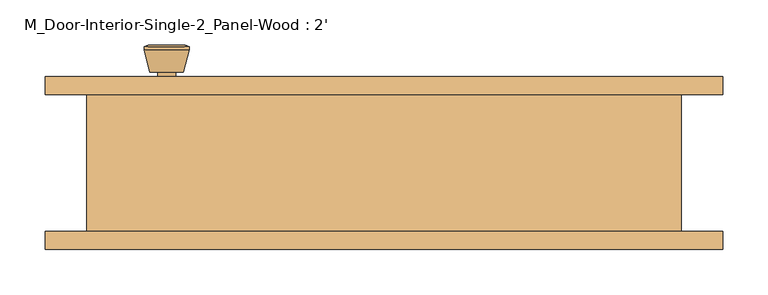
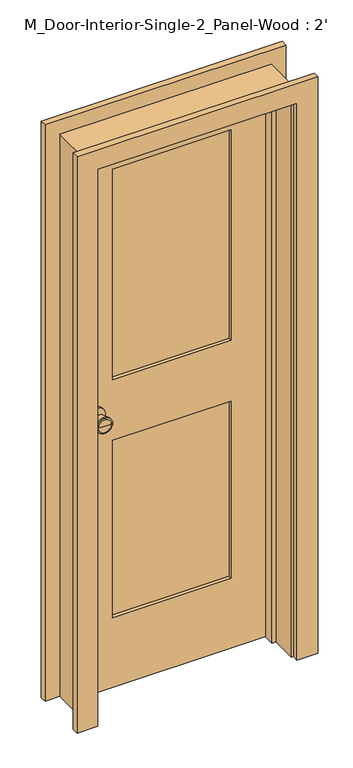
"""IFC4 building model written with IfcOpenShell, lengths in millimetres: door geometry, M_Door-Interior-Single-2_Panel-Wood : 2'."""

from ifc_helpers import new_model, si_unit, point, frame, frame_2d, origin, place, context, project, spatial, polyline, circle_curve, trimmed, segment, composite_curve, outline, extrude, faceted_brep, source, transform, mapped, element, save
from ifc_brep_helpers import plane_surface, cylinder_surface, revolved_surface, advanced_brep


def m_door_interior_single_2_panel_wood_2_8c5b34de(model_context):
    return source(origin(), model_context, "Body", "SolidModel", [
        advanced_brep(
        [(-241.3, 32.025, 914.4), (-231.3, 32.025, 914.4), (-251.3, 32.025, 914.4), (-220.8241324, -16.975, 914.4), (-241.3, -16.975, 914.4), (-261.7758676, -16.975, 914.4), (-216.3, -15.1471319, 914.4), (-266.3, -15.1471319, 914.4), (-216.3, -11.6834537, 914.4), (-266.3, -11.6834537, 914.4), (-222.663764, 13.025, 914.4), (-259.936236, 13.025, 914.4), (-231.3, 13.025, 914.4), (-251.3, 13.025, 914.4)],
        [
            (0, 1),
            (1, 2, circle_curve(frame((-241.3, 32.025, 914.4), z_axis=(0.0, 1.0, 0.0), x_axis=(-1.0, 0.0, 0.0)), 10.0)),
            (2, 0),
            (2, 1, circle_curve(frame((-241.3, 32.025, 914.4), z_axis=(0.0, 1.0, 0.0), x_axis=(-1.0, 0.0, 0.0)), 10.0)),
            (3, 4),
            (4, 5),
            (5, 3, circle_curve(frame((-241.3, -16.975, 914.4), z_axis=(0.0, -1.0, 0.0), x_axis=(-1.0, 0.0, 0.0)), 20.4758676)),
            (3, 5, circle_curve(frame((-241.3, -16.975, 914.4), z_axis=(0.0, -1.0, 0.0), x_axis=(-1.0, 0.0, 0.0)), 20.4758676)),
            (6, 3),
            (5, 7),
            (7, 6, circle_curve(frame((-241.3, -15.1471319, 914.4), z_axis=(0.0, -1.0, 0.0), x_axis=(-1.0, 0.0, 0.0)), 25.0)),
            (6, 7, circle_curve(frame((-241.3, -15.1471319, 914.4), z_axis=(0.0, -1.0, 0.0), x_axis=(-1.0, 0.0, 0.0)), 25.0)),
            (8, 6),
            (7, 9),
            (9, 8, circle_curve(frame((-241.3, -11.6834537, 914.4), z_axis=(0.0, -1.0, 0.0), x_axis=(-1.0, 0.0, 0.0)), 25.0)),
            (8, 9, circle_curve(frame((-241.3, -11.6834537, 914.4), z_axis=(0.0, -1.0, 0.0), x_axis=(-1.0, 0.0, 0.0)), 25.0)),
            (10, 8),
            (9, 11),
            (11, 10, circle_curve(frame((-241.3, 13.025, 914.4), z_axis=(0.0, -1.0, 0.0), x_axis=(-1.0, 0.0, 0.0)), 18.636236)),
            (10, 11, circle_curve(frame((-241.3, 13.025, 914.4), z_axis=(0.0, -1.0, 0.0), x_axis=(-1.0, 0.0, 0.0)), 18.636236)),
            (12, 10),
            (11, 13),
            (13, 12, circle_curve(frame((-241.3, 13.025, 914.4), z_axis=(0.0, -1.0, 0.0), x_axis=(-1.0, 0.0, 0.0)), 10.0)),
            (12, 13, circle_curve(frame((-241.3, 13.025, 914.4), z_axis=(0.0, -1.0, 0.0), x_axis=(-1.0, 0.0, 0.0)), 10.0)),
            (1, 12),
            (13, 2),
        ],
        [
            plane_surface(frame((-241.3, 32.025, 914.4), z_axis=(0.0, 1.0, 0.0), x_axis=(-1.0, 0.0, 0.0))),
            plane_surface(frame((-241.3, -16.975, 914.4), z_axis=(0.0, -1.0, 0.0), x_axis=(-1.0, 0.0, 0.0))),
            revolved_surface(polyline([(-261.7758676, -16.975, 914.4), (-266.3, -15.1471319, 914.4)]), (-241.3, 32.025, 914.4), (0.0, 1.0, 0.0)),
            cylinder_surface(frame((-241.3, 32.025, 914.4), z_axis=(0.0, 1.0, 0.0), x_axis=(-1.0, 0.0, 0.0)), 25.0),
            revolved_surface(polyline([(-266.3, -11.6834537, 914.4), (-259.936236, 13.025, 914.4)]), (-241.3, 32.025, 914.4), (0.0, 1.0, 0.0)),
            plane_surface(frame((-241.3, 13.025, 914.4), z_axis=(0.0, 1.0, 0.0), x_axis=(-1.0, 0.0, 0.0))),
            cylinder_surface(frame((-241.3, 32.025, 914.4), z_axis=(0.0, 1.0, 0.0), x_axis=(-1.0, 0.0, 0.0)), 10.0),
        ],
        [
            (0, [[1, 2, 3]]),
            (0, [[-3, 4, -1]]),
            (1, [[5, 6, 7]]),
            (1, [[-6, -5, 8]]),
            (2, [[9, -7, 10, 11]]),
            (2, [[-10, -8, -9, 12]]),
            (3, [[13, -11, 14, 15]]),
            (3, [[-14, -12, -13, 16]]),
            (4, [[17, -15, 18, 19]]),
            (4, [[-18, -16, -17, 20]]),
            (5, [[21, -19, 22, 23]]),
            (5, [[-22, -20, -21, 24]]),
            (6, [[25, -23, 26, -2]]),
            (6, [[-26, -24, -25, -4]]),
        ],
    ),
        extrude(outline(composite_curve([segment(trimmed(circle_curve(frame_2d((914.4, -241.3)), 30.0), [point((914.4, -271.3))], [point((914.4, -211.3))], False, "CARTESIAN"), True, "CONTINUOUS"), segment(trimmed(circle_curve(frame_2d((914.4, -241.3)), 30.0), [point((914.4, -211.3))], [point((914.4, -271.3))], False, "CARTESIAN"), True, "CONTINUOUS")], self_intersect=False)), frame((0.0, 32.025, 0.0), z_axis=(0.0, 1.0, 0.0), x_axis=(0.0, 0.0, 1.0)), (0.0, 0.0, 1.0), 6.0),
        advanced_brep(
        [(-241.3, 79.025, 914.4), (-251.3, 79.025, 914.4), (-231.3, 79.025, 914.4), (-220.8241324, 128.025, 914.4), (-261.7758676, 128.025, 914.4), (-241.3, 128.025, 914.4), (-216.3, 126.1971319, 914.4), (-266.3, 126.1971319, 914.4), (-216.3, 122.7334537, 914.4), (-266.3, 122.7334537, 914.4), (-222.663764, 98.025, 914.4), (-259.936236, 98.025, 914.4), (-231.3, 98.025, 914.4), (-251.3, 98.025, 914.4)],
        [
            (0, 1),
            (1, 2, circle_curve(frame((-241.3, 79.025, 914.4), z_axis=(0.0, -1.0, 0.0), x_axis=(-1.0, 0.0, 0.0)), 10.0)),
            (2, 0),
            (2, 1, circle_curve(frame((-241.3, 79.025, 914.4), z_axis=(0.0, -1.0, 0.0), x_axis=(-1.0, 0.0, 0.0)), 10.0)),
            (3, 4, circle_curve(frame((-241.3, 128.025, 914.4), z_axis=(0.0, 1.0, 0.0), x_axis=(-1.0, 0.0, 0.0)), 20.4758676)),
            (4, 5),
            (5, 3),
            (4, 3, circle_curve(frame((-241.3, 128.025, 914.4), z_axis=(0.0, 1.0, 0.0), x_axis=(-1.0, 0.0, 0.0)), 20.4758676)),
            (6, 7, circle_curve(frame((-241.3, 126.1971319, 914.4), z_axis=(0.0, 1.0, 0.0), x_axis=(-1.0, 0.0, 0.0)), 25.0)),
            (7, 4),
            (3, 6),
            (7, 6, circle_curve(frame((-241.3, 126.1971319, 914.4), z_axis=(0.0, 1.0, 0.0), x_axis=(-1.0, 0.0, 0.0)), 25.0)),
            (8, 9, circle_curve(frame((-241.3, 122.7334537, 914.4), z_axis=(0.0, 1.0, 0.0), x_axis=(-1.0, 0.0, 0.0)), 25.0)),
            (9, 7),
            (6, 8),
            (9, 8, circle_curve(frame((-241.3, 122.7334537, 914.4), z_axis=(0.0, 1.0, 0.0), x_axis=(-1.0, 0.0, 0.0)), 25.0)),
            (10, 11, circle_curve(frame((-241.3, 98.025, 914.4), z_axis=(0.0, 1.0, 0.0), x_axis=(-1.0, 0.0, 0.0)), 18.636236)),
            (11, 9),
            (8, 10),
            (11, 10, circle_curve(frame((-241.3, 98.025, 914.4), z_axis=(0.0, 1.0, 0.0), x_axis=(-1.0, 0.0, 0.0)), 18.636236)),
            (12, 13, circle_curve(frame((-241.3, 98.025, 914.4), z_axis=(0.0, 1.0, 0.0), x_axis=(-1.0, 0.0, 0.0)), 10.0)),
            (13, 11),
            (10, 12),
            (13, 12, circle_curve(frame((-241.3, 98.025, 914.4), z_axis=(0.0, 1.0, 0.0), x_axis=(-1.0, 0.0, 0.0)), 10.0)),
            (1, 13),
            (12, 2),
        ],
        [
            plane_surface(frame((-241.3, 79.025, 914.4), z_axis=(0.0, -1.0, 0.0), x_axis=(-1.0, 0.0, 0.0))),
            plane_surface(frame((-241.3, 128.025, 914.4), z_axis=(0.0, 1.0, 0.0), x_axis=(-1.0, 0.0, 0.0))),
            revolved_surface(polyline([(-261.7758676, 128.025, 914.4), (-266.3, 126.1971319, 914.4)]), (-241.3, 79.025, 914.4), (0.0, -1.0, 0.0)),
            cylinder_surface(frame((-241.3, 79.025, 914.4), z_axis=(0.0, -1.0, 0.0), x_axis=(-1.0, 0.0, 0.0)), 25.0),
            revolved_surface(polyline([(-266.3, 122.7334537, 914.4), (-259.936236, 98.025, 914.4)]), (-241.3, 79.025, 914.4), (0.0, -1.0, 0.0)),
            plane_surface(frame((-241.3, 98.025, 914.4), z_axis=(0.0, -1.0, 0.0), x_axis=(-1.0, 0.0, 0.0))),
            cylinder_surface(frame((-241.3, 79.025, 914.4), z_axis=(0.0, -1.0, 0.0), x_axis=(-1.0, 0.0, 0.0)), 10.0),
        ],
        [
            (0, [[1, 2, 3]]),
            (0, [[-3, 4, -1]]),
            (1, [[5, 6, 7]]),
            (1, [[8, -7, -6]]),
            (2, [[9, 10, -5, 11]]),
            (2, [[12, -11, -8, -10]]),
            (3, [[13, 14, -9, 15]]),
            (3, [[16, -15, -12, -14]]),
            (4, [[17, 18, -13, 19]]),
            (4, [[20, -19, -16, -18]]),
            (5, [[21, 22, -17, 23]]),
            (5, [[24, -23, -20, -22]]),
            (6, [[-2, 25, -21, 26]]),
            (6, [[-4, -26, -24, -25]]),
        ],
    ),
        extrude(outline(composite_curve([segment(trimmed(circle_curve(frame_2d((914.4, -241.3)), 30.0), [point((914.4, -271.3))], [point((914.4, -211.3))], False, "CARTESIAN"), True, "CONTINUOUS"), segment(trimmed(circle_curve(frame_2d((914.4, -241.3)), 30.0), [point((914.4, -211.3))], [point((914.4, -271.3))], False, "CARTESIAN"), True, "CONTINUOUS")], self_intersect=False)), frame((0.0, 73.025, 0.0), z_axis=(0.0, 1.0, 0.0), x_axis=(0.0, 0.0, 1.0)), (0.0, 0.0, 1.0), 6.0),
        faceted_brep([(329.8, 73.025, 0.0), (329.8, -79.375, 0.0), (304.8, -79.375, 0.0), (304.8, 3.1, 0.0), (292.1, 3.1, 0.0), (292.1, 38.025, 0.0), (304.8, 38.025, 0.0), (304.8, 73.025, 0.0), (329.8, 73.025, 1853.8), (329.8, -79.375, 1853.8), (-329.8, -79.375, 1853.8), (-329.8, -79.375, 0.0), (-304.8, -79.375, 0.0), (-304.8, -79.375, 1828.8), (304.8, -79.375, 1828.8), (304.8, 3.1, 1828.8), (-304.8, 3.1, 1828.8), (-304.8, 3.1, 0.0), (-292.1, 3.1, 0.0), (-292.1, 3.1, 1816.1), (292.1, 3.1, 1816.1), (292.1, 38.025, 1816.1), (-292.1, 38.025, 1816.1), (-292.1, 38.025, 0.0), (-304.8, 38.025, 0.0), (-304.8, 38.025, 1828.8), (304.8, 38.025, 1828.8), (304.8, 73.025, 1828.8), (-304.8, 73.025, 1828.8), (-304.8, 73.025, 0.0), (-329.8, 73.025, 0.0), (-329.8, 73.025, 1853.8)], [[[0, 1, 2, 3, 4, 5, 6, 7]], [[1, 0, 8, 9]], [[2, 1, 9, 10, 11, 12, 13, 14]], [[3, 2, 14, 15]], [[4, 3, 15, 16, 17, 18, 19, 20]], [[5, 4, 20, 21]], [[6, 5, 21, 22, 23, 24, 25, 26]], [[7, 6, 26, 27]], [[0, 7, 27, 28, 29, 30, 31, 8]], [[9, 8, 31, 10]], [[15, 14, 13, 16]], [[21, 20, 19, 22]], [[27, 26, 25, 28]], [[30, 29, 24, 23, 18, 17, 12, 11]], [[10, 31, 30, 11]], [[16, 13, 12, 17]], [[22, 19, 18, 23]], [[28, 25, 24, 29]]]),
        extrude(outline(polyline([(1828.8, -304.8), (0.0, -304.8), (0.0, 304.8), (1828.8, 304.8), (1828.8, -304.8)]), holes=[polyline([(1708.8, -184.8), (1708.8, 184.8), (1014.4, 184.8), (1014.4, -184.8), (1708.8, -184.8)]), polyline([(814.4, -184.8), (814.4, 184.8), (230.0, 184.8), (230.0, -184.8), (814.4, -184.8)])]), frame((0.0, 38.025, 0.0), z_axis=(0.0, 1.0, 0.0), x_axis=(0.0, 0.0, 1.0)), (0.0, 0.0, 1.0), 35.0),
        extrude(outline(polyline([(184.8, 49.6916667), (-184.8, 49.6916667), (-184.8, 61.3583333), (184.8, 61.3583333), (184.8, 49.6916667)])), frame((0.0, 0.0, 1014.4), z_axis=(0.0, 0.0, 1.0), x_axis=(1.0, 0.0, 0.0)), (0.0, 0.0, 1.0), 694.4),
        extrude(outline(polyline([(184.8, 49.6916667), (-184.8, 49.6916667), (-184.8, 61.3583333), (184.8, 61.3583333), (184.8, 49.6916667)])), frame((0.0, 0.0, 230.0), z_axis=(0.0, 0.0, 1.0), x_axis=(1.0, 0.0, 0.0)), (0.0, 0.0, 1.0), 584.4),
        extrude(outline(polyline([(0.0, 311.15), (0.0, 376.15), (1900.15, 376.15), (1900.15, -376.15), (0.0, -376.15), (0.0, -311.15), (1835.15, -311.15), (1835.15, 311.15), (0.0, 311.15)])), frame((0.0, 73.025, 0.0), z_axis=(0.0, 1.0, 0.0), x_axis=(0.0, 0.0, 1.0)), (0.0, 0.0, 1.0), 20.0),
        extrude(outline(polyline([(0.0, 311.15), (0.0, 376.15), (1900.15, 376.15), (1900.15, -376.15), (0.0, -376.15), (0.0, -311.15), (1835.15, -311.15), (1835.15, 311.15), (0.0, 311.15)])), frame((0.0, -99.375, 0.0), z_axis=(0.0, 1.0, 0.0), x_axis=(0.0, 0.0, 1.0)), (0.0, 0.0, 1.0), 20.0),
    ])


if __name__ == "__main__":
    model = new_model("IFC4")
    model_context = context("Model", 3, world=origin())
    ifc_project = project(units=[si_unit("LENGTHUNIT", "METRE", prefix="MILLI")], contexts=[model_context])
    site = spatial("IfcSite", under=ifc_project)
    building = spatial("IfcBuilding", under=site)
    placement = place(None, origin())
    m_door_interior_single_2_panel_wood_2_shape = m_door_interior_single_2_panel_wood_2_8c5b34de(model_context)
    element("IfcDoor", 1, ObjectType="M_Door-Interior-Single-2_Panel-Wood : 2'", at=placement, inside=building, context=model_context, shape_type="MappedRepresentation", body=[
        mapped(m_door_interior_single_2_panel_wood_2_shape, transform((0.0, 0.0, 0.0), x_axis=(1.0, 0.0, 0.0), y_axis=(0.0, 1.0, 0.0), z_axis=(0.0, 0.0, 1.0))),
    ])
    save(model, "model.ifc")

# Revit data of these elements
# Type "M_Door-Interior-Single-2_Panel-Wood : 2'"
#   Type Mark = "12"
#   Assembly Code = "C1020300"
#   Analytic Construction = "Wooden"
#   Top Rail = 0' - 4.72441"
#   Thickness = 0' - 1.37795"
#   Thermal Resistance (R) = 2.5876 (h·ft²·°F)/BTU
#   Swing Angle [instance default] = 90.00°
#   Stiles = 0' - 4.72441"
#   Rough Width = 2' - 1.9685"
#   Rough Height = 6' - 0.98425"
#   Lock Rail = 0' - 7.87402"
#   Height = 6' - 0"
#   Width = 2' - 0"
#   Heat Transfer Coefficient (U) = 0.3865 BTU/(h·ft²·°F)
#   Bottom Rail = 0' - 9.05512"
#   Trim Material = Cherry
#   Panel Material = Cherry
#   Frame Material = Cherry
#   Door Handle Material = Aluminum
#   Visual Light Transmittance = 0
#   Solar Heat Gain Coefficient = 0
#   Wall Closure = (empty or 0)
#   Function = (empty or 0)
# Element 1 (IfcDoor, "M_Door-Interior-Single-2_Panel-Wood : 2'")
#   Materials on its faces: "Cherry", "Aluminum"
# Materials
#   "Cherry": class "Wood", colour RGB 226 177 128, transparency 0, Description = "Prunus Serotina", Cost = 0
#   "Aluminum": class "Metal", colour RGB 247 247 247, transparency 0, Description = "Aluminum 6061", Cost = 0
